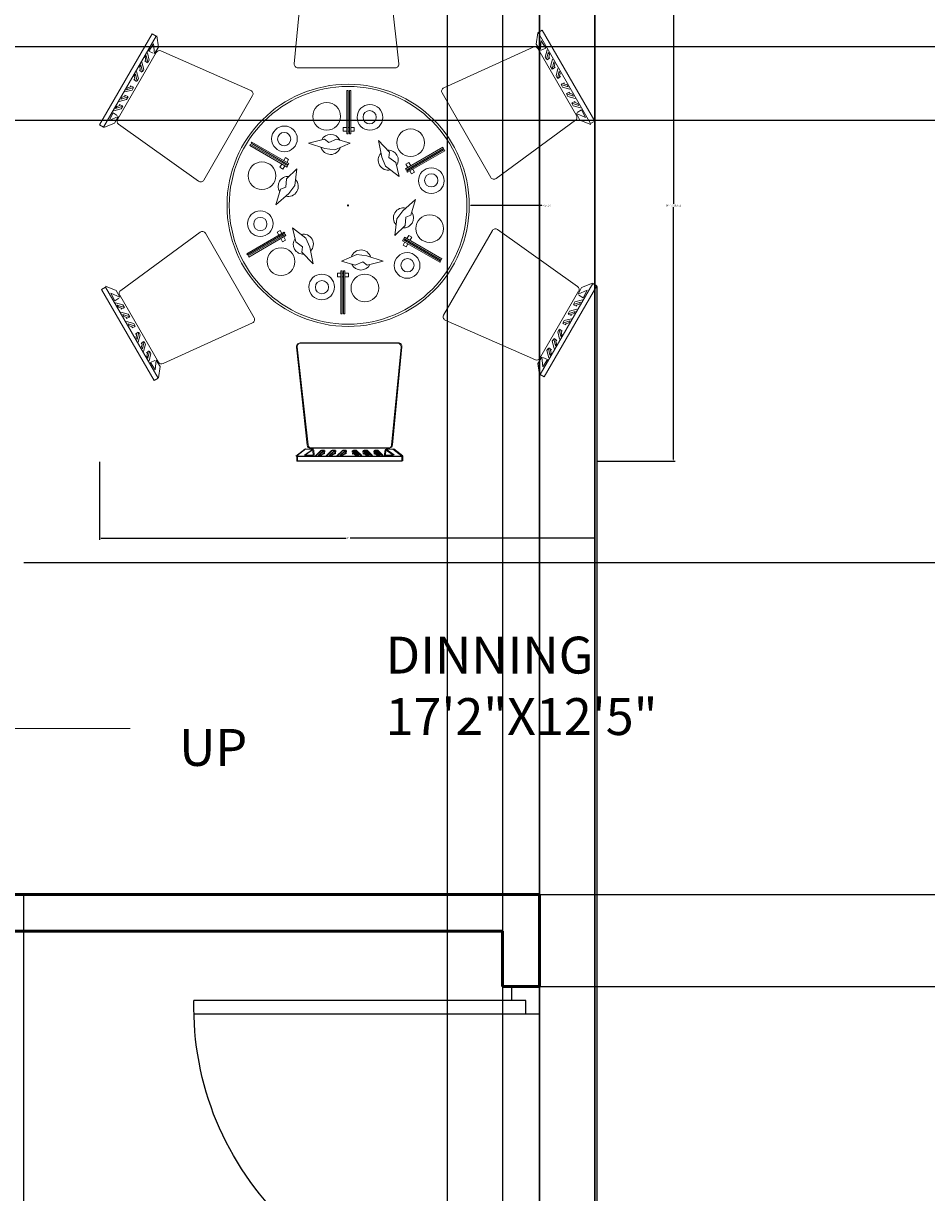
# Model space of a CAD drawing. Units: inches. Extents: x 1798 to 2141, y 1923 to 2386.
# Tile 3 of 9: x 1921 to 2019, y 2050 to 2177. Entities that reach past the tile are written whole.
import ezdxf

# ---------------------------------------------------------------- set-up
doc = ezdxf.new("R2010")
doc.units = ezdxf.units.IN
for name, color, linetype, lineweight in [('A-ANNO-DIMS', 2, 'Continuous', 18), ('A-ANNO-SYMB', 7, 'Continuous', 18), ('A-ANNO-TEXT', 7, 'Continuous', 18), ('A-AREA-IDEN', 7, 'Continuous', 25), ('A-FURN', 8, 'Continuous', 13), ('door', 40, 'Continuous', 25), ('wall', 4, 'Continuous', 50)]:
    doc.layers.add(name, color=color, linetype=linetype, lineweight=lineweight)
doc.styles.get("Standard").update_dxf_attribs({"font": 'arial.ttf'})
doc.dimstyles.get("Standard").update_dxf_attribs({"dimtxt": 0.18, "dimasz": 0.18, "dimexe": 0.18, "dimexo": 0.0625, "dimgap": 0.09, "dimtad": 0, "dimtih": 1, "dimtoh": 1, "dimdec": 4, "dimzin": 0, "dimdsep": 46, "dimtxsty": 'Standard', "dimcen": 0.09, "dimadec": 0, "dimazin": 0, "dimtfac": 1, "dimtdec": 4, "dimtofl": 0, "dimtmove": 0, "dimatfit": 3, "dimfxl": 1, "dimtolj": 1, "dimtzin": 0, "dimarcsym": 0})

# ---------------------------------------------------------------- blocks, each defined once
blk = doc.blocks.new('A$C45501D90')
for p, q in [((-242.2, 1133.5), (224, 1133.5)), ((-242.2, 1112.8), (-242.2, 1133.5)), ((224, 1112.8), (-242.2, 1112.8)), ((-242.2, 1111.2), (-202.3, 1079.2)), ((-203.9, 1106.4), (-165.6, 1108)), ((-168.8, 1080.8), (-203.9, 1106.4)), ((-165.6, 1108), (-167.2, 1085.6)), ((-156, 1109.6), (-132, 1085.6)), ((-119.3, 1085.6), (-143.2, 1108)), ((-143.2, 1108), (-133.6, 1108)), ((-133.6, 1108), (-122.5, 1098.4)), ((-122.5, 1098.4), (-119.3, 1101.6)), ((-119.3, 1101.6), (-117.7, 1087.2)), ((-108.1, 1109.6), (-84.1, 1085.6)), ((-71.4, 1085.6), (-95.3, 1108)), ((-95.3, 1108), (-85.7, 1108)), ((-85.7, 1108), (-74.6, 1098.4)), ((-74.6, 1098.4), (-71.4, 1101.6)), ((-71.4, 1101.6), (-69.8, 1087.2)), ((-60.2, 1109.6), (-36.2, 1085.6)), ((-23.5, 1085.6), (-47.4, 1108)), ((-47.4, 1108), (-37.8, 1108)), ((-37.8, 1108), (-26.7, 1098.4)), ((-26.7, 1098.4), (-23.5, 1101.6)), ((-23.5, 1101.6), (-21.9, 1087.2)), ((8.5, 1101.6), (6.9, 1087.2)), ((8.5, 1085.6), (32.4, 1108)), ((11.6, 1098.4), (8.5, 1101.6)), ((22.8, 1108), (11.6, 1098.4)), ((45.2, 1109.6), (21.2, 1085.6)), ((32.4, 1108), (22.8, 1108)), ((56.3, 1101.6), (54.8, 1087.2)), ((56.3, 1085.6), (80.3, 1108)), ((59.5, 1098.4), (56.3, 1101.6)), ((70.7, 1108), (59.5, 1098.4)), ((93.1, 1109.6), (69.1, 1085.6)), ((80.3, 1108), (70.7, 1108)), ((104.2, 1101.6), (102.6, 1087.2)), ((104.2, 1085.6), (128.2, 1108)), ((107.4, 1098.4), (104.2, 1101.6)), ((118.6, 1108), (107.4, 1098.4)), ((141, 1109.6), (117, 1085.6)), ((128.2, 1108), (118.6, 1108)), ((188.9, 1106.4), (150.5, 1108)), ((150.5, 1108), (152.1, 1085.6)), ((153.7, 1080.8), (188.9, 1106.4)), ((224, 1112.8), (187.3, 1079.2)), ((224, 1133.5), (224, 1112.8)), ((-197.3, 1061.6), (-238.9, 627.6)), ((-202.3, 1079.2), (-168.8, 1080.8)), ((161.8, 1076.1), (-181.4, 1076.1)), ((-132, 1085.6), (-119.3, 1085.6)), ((-84.1, 1085.6), (-71.4, 1085.6)), ((-36.2, 1085.6), (-23.5, 1085.6)), ((21.2, 1085.6), (8.5, 1085.6)), ((69.1, 1085.6), (56.3, 1085.6)), ((117, 1085.6), (104.2, 1085.6)), ((187.3, 1079.2), (153.7, 1080.8)), ((225.2, 627.8), (177.6, 1061.8)), ((-1102.7, 357), (-869.7, 760.7)), ((-851.7, 750.4), (-1084.8, 346.6)), ((-869.7, 760.7), (-851.7, 750.4)), ((-848.7, 752.3), (-841, 701.8)), ((841.2, 765.3), (833.5, 714.8)), ((842.6, 766.1), (860.5, 776.5)), ((1075.7, 362.4), (842.6, 766.1)), ((851.7, 686.6), (856.2, 729.8)), ((856.2, 729.8), (876.7, 697.4)), ((860.5, 776.5), (1093.6, 372.8)), ((-851, 678.1), (-1022.6, 380.9)), ((-890.4, 676.9), (-881.7, 644.2)), ((-863.7, 716.7), (-884.3, 684.4)), ((-884.3, 684.4), (-864.1, 674.6)), ((-859.2, 673.6), (-863.7, 716.7)), ((-841, 701.8), (-859.2, 673.6)), ((-431.1, 509), (-830.8, 684.8)), ((820.7, 701.7), (424.1, 520.7)), ((833.5, 714.8), (851.7, 686.6)), ((1012.8, 397.9), (841.2, 695.1)), ((876.7, 697.4), (856.6, 687.6)), ((882.9, 689.9), (874.2, 657.2)), ((880.6, 646.1), (887.9, 678)), ((887.9, 678), (892.7, 669.7)), ((-919.4, 623.5), (-924.2, 615.2)), ((-912, 591.6), (-919.4, 623.5)), ((-914.4, 635.4), (-905.6, 602.7)), ((-897.5, 642.2), (-901.9, 641.1)), ((-901.9, 641.1), (-890.2, 632.5)), ((-895.4, 665), (-900.2, 656.7)), ((-900.2, 656.7), (-897.5, 642.2)), ((-888.1, 633.1), (-895.4, 665)), ((-881.7, 644.2), (-888.1, 633.1)), ((874.2, 657.2), (880.6, 646.1)), ((894.4, 654.1), (882.7, 645.5)), ((892.7, 669.7), (890, 655.2)), ((890, 655.2), (894.4, 654.1)), ((906.9, 648.4), (898.1, 615.7)), ((904.5, 604.6), (911.9, 636.5)), ((911.9, 636.5), (916.7, 628.2)), ((916.7, 628.2), (914, 613.8)), ((-943.3, 582), (-948.1, 573.8)), ((-948.1, 573.8), (-945.4, 559.3)), ((-936, 550.1), (-943.3, 582)), ((-938.3, 593.9), (-929.6, 561.2)), ((-921.5, 600.8), (-925.8, 599.6)), ((-925.8, 599.6), (-914.2, 591)), ((-924.2, 615.2), (-921.5, 600.8)), ((-905.6, 602.7), (-912, 591.6)), ((-223, 610.1), (209.4, 610.1)), ((898.1, 615.7), (904.5, 604.6)), ((918.3, 612.6), (906.7, 604)), ((914, 613.8), (918.3, 612.6)), ((930.8, 606.9), (922.1, 574.2)), ((922.1, 574.2), (928.4, 563.1)), ((928.4, 563.1), (935.8, 595.1)), ((942.3, 571.1), (930.6, 562.6)), ((935.8, 595.1), (940.6, 586.8)), ((940.6, 586.8), (937.9, 572.3)), ((937.9, 572.3), (942.3, 571.1)), ((-951.9, 522.5), (-983.2, 512.9)), ((-983.2, 512.9), (-978.5, 521.2)), ((-978.5, 521.2), (-964.6, 526.1)), ((-964.6, 526.1), (-965.7, 530.5)), ((-965.7, 530.5), (-952.5, 524.7)), ((-958.3, 511.4), (-951.9, 522.5)), ((-945.4, 559.3), (-949.8, 558.1)), ((-949.8, 558.1), (-938.1, 549.6)), ((-929.6, 561.2), (-936, 550.1)), ((950.8, 524.4), (944.4, 535.5)), ((944.4, 535.5), (975.7, 525.9)), ((958.2, 543.5), (945, 537.7)), ((983.5, 515.7), (950.8, 524.4)), ((957.1, 539.1), (958.2, 543.5)), ((970.9, 534.2), (957.1, 539.1)), ((975.7, 525.9), (970.9, 534.2)), ((-1015, 461.2), (-982.3, 469.9)), ((-975.9, 481), (-1007.2, 471.4)), ((-1007.2, 471.4), (-1002.4, 479.7)), ((-1002.4, 479.7), (-988.5, 484.6)), ((-991, 502.7), (-958.3, 511.4)), ((-988.5, 484.6), (-989.7, 489)), ((-989.7, 489), (-976.5, 483.2)), ((-982.3, 469.9), (-975.9, 481)), ((-639.9, 111.9), (-423.7, 486.4)), ((-5.6, 508.7, 90.8), (0.4, 508.7, 90.8)), ((-5.6, 317.7, 90.8), (-5.6, 508.7, 90.8)), ((0.4, 508.7, 90.8), (0.4, 317.7, 90.8)), ((5.8, 317.7, 90.8), (5.8, 508.7, 90.8)), ((5.8, 508.7, 90.8), (11.8, 508.7, 90.8)), ((11.8, 508.7, 90.8), (11.8, 317.7, 90.8)), ((416.9, 498.2), (633.1, 123.7)), ((968.4, 494), (999.7, 484.4)), ((974.7, 483), (968.4, 494)), ((982.2, 502), (968.9, 496.2)), ((1007.4, 474.2), (974.7, 483)), ((981, 497.6), (982.2, 502)), ((994.9, 492.7), (981, 497.6)), ((999.7, 484.4), (994.9, 492.7)), ((-1038.9, 419.7), (-1006.2, 428.5)), ((-999.8, 439.5), (-1031.1, 430)), ((-1031.1, 430), (-1026.3, 438.3)), ((-1026.3, 438.3), (-1012.5, 443.1)), ((-1012.5, 443.1), (-1013.6, 447.5)), ((-1013.6, 447.5), (-1000.4, 441.7)), ((-1006.2, 428.5), (-999.8, 439.5)), ((998.7, 441.5), (992.3, 452.5)), ((992.3, 452.5), (1023.6, 443)), ((1006.1, 460.5), (992.9, 454.7)), ((1031.4, 432.7), (998.7, 441.5)), ((1005, 456.2), (1006.1, 460.5)), ((1018.8, 451.3), (1005, 456.2)), ((1034.8, 423.6), (1016.3, 411.1)), ((1023.6, 443), (1018.8, 451.3)), ((1052.6, 389.6), (1034.8, 423.6)), ((-1083.4, 345.8), (-1035.8, 364.4)), ((-1060.1, 376.6), (-1042.3, 410.6)), ((-1020.4, 394.3), (-1060.1, 376.6)), ((-1042.3, 410.6), (-1023.8, 398.1)), ((-1035.8, 364.4), (-1020.4, 394.3)), ((656.3, 118.9), (1008.4, 377.1)), ((1028.3, 377.5), (1012.9, 407.3)), ((1012.9, 407.3), (1052.6, 389.6)), ((1075.9, 358.8), (1028.3, 377.5)), ((1093.6, 372.8), (1075.7, 362.4)), ((-1084.8, 346.6), (-1102.7, 357)), ((-1018, 360), (-663, 106.9)), ((-22.3, 329.1, 90.8), (-22.3, 344.6, 90.8)), ((-22.3, 344.6, 90.8), (-5.6, 344.6, 90.8)), ((-5.6, 329.1, 90.8), (-22.3, 329.1, 90.8)), ((0.4, 317.7, 90.8), (-5.6, 317.7, 90.8)), ((0.4, 344.6, 90.8), (5.8, 344.6, 90.8)), ((5.8, 329.1, 90.8), (0.4, 329.1, 90.8)), ((11.8, 317.7, 90.8), (5.8, 317.7, 90.8)), ((11.8, 344.6, 90.8), (27.3, 344.6, 90.8)), ((27.3, 329.1, 90.8), (11.8, 329.1, 90.8)), ((27.3, 344.6, 90.8), (27.3, 329.1, 90.8)), ((-436.3, 265.3, 90.8), (-433.3, 270.5, 90.8)), ((-270.9, 169.9, 90.8), (-436.3, 265.3, 90.8)), ((-433.3, 270.5, 90.8), (-267.9, 175, 90.8)), ((-430.6, 275.2, 90.8), (-427.6, 280.3, 90.8)), ((-265.2, 179.7, 90.8), (-430.6, 275.2, 90.8)), ((-427.6, 280.3, 90.8), (-262.3, 184.9, 90.8)), ((-175.3, 276.1, 90.8), (-104.8, 293.2, 90.8)), ((-103.3, 252.4, 90.8), (-175.3, 276.1, 90.8)), ((-104.8, 293.2, 90.8), (-85.5, 278.4, 90.8)), ((-85.5, 278.4, 90.8), (-52.1, 293.9, 90.8)), ((9.5, 276.1, 90.8), (-59.5, 246.5, 90.8)), ((-52.1, 293.9, 90.8), (9.5, 276.1, 90.8)), ((134.3, 288, 90.8), (184.3, 235.5, 90.8)), ((149.7, 213.9, 90.8), (134.3, 288, 90.8)), ((-285.5, 198.3, 90.8), (-277.8, 211.7, 90.8)), ((-277.8, 211.7, 90.8), (-264.3, 204, 90.8)), ((-59.5, 246.5, 90.8), (-103.3, 252.4, 90.8)), ((166.5, 173, 90.8), (149.7, 213.9, 90.8)), ((184.3, 235.5, 90.8), (181.1, 211.4, 90.8)), ((181.1, 211.4, 90.8), (211.3, 190.3, 90.8)), ((255.2, 161.9, 90.8), (420.6, 257.3, 90.8)), ((423.5, 252.2, 90.8), (258.2, 156.7, 90.8)), ((260.9, 152, 90.8), (426.2, 247.5, 90.8)), ((429.2, 242.3, 90.8), (263.8, 146.9, 90.8)), ((420.6, 257.3, 90.8), (423.5, 252.2, 90.8)), ((426.2, 247.5, 90.8), (429.2, 242.3, 90.8)), ((-302.5, 168.8, 90.8), (-294.2, 183.3, 90.8)), ((-289.1, 161.1, 90.8), (-302.5, 168.8, 90.8)), ((-291.2, 188.5, 90.8), (-288.5, 193.1, 90.8)), ((-280.7, 175.5, 90.8), (-289.1, 161.1, 90.8)), ((-275.1, 185.4, 90.8), (-277.8, 180.7, 90.8)), ((-273.6, 117.6, 90.8), (-227.4, 162.1, 90.8)), ((-264.3, 204, 90.8), (-272.1, 190.5, 90.8)), ((-267.9, 175, 90.8), (-270.9, 169.9, 90.8)), ((-262.3, 184.9, 90.8), (-265.2, 179.7, 90.8)), ((-227.4, 162.1, 90.8), (-236.2, 87.5, 90.8)), ((226.7, 128.1, 90.8), (166.5, 173, 90.8)), ((211.3, 190.3, 90.8), (226.7, 128.1, 90.8)), ((258.2, 156.7, 90.8), (255.2, 161.9, 90.8)), ((256.6, 182, 90.8), (270.1, 189.8, 90.8)), ((265, 167.5, 90.8), (256.6, 182, 90.8)), ((270.7, 157.7, 90.8), (268, 162.4, 90.8)), ((270.1, 189.8, 90.8), (278.4, 175.3, 90.8)), ((281.4, 170.1, 90.8), (284.1, 165.5, 90.8)), ((287.1, 160.3, 90.8), (294.9, 146.8, 90.8)), ((-276.8, 80.9, 90.8), (-273.6, 117.6, 90.8)), ((263.8, 146.9, 90.8), (260.9, 152, 90.8)), ((281.4, 139.1, 90.8), (273.7, 152.5, 90.8)), ((294.9, 146.8, 90.8), (281.4, 139.1, 90.8)), ((-319.8, 2.1, 90.8), (-299.3, 71.7, 90.8)), ((-263.2, 52.5, 90.8), (-319.8, 2.1, 90.8)), ((-299.3, 71.7, 90.8), (-276.8, 80.9, 90.8)), ((-236.2, 87.5, 90.8), (-263.2, 52.5, 90.8)), ((242.9, -24.6, 90.8), (299.4, 25.9, 90.8)), ((299.4, 25.9, 90.8), (278.9, -43.7, 90.8)), ((215.8, -59.5, 90.8), (242.9, -24.6, 90.8)), ((278.9, -43.7, 90.8), (256.4, -53, 90.8)), ((-247, -100.1, 90.8), (-186.8, -145, 90.8)), ((-231.7, -162.3, 90.8), (-247, -100.1, 90.8)), ((207, -134.1, 90.8), (215.8, -59.5, 90.8)), ((253.2, -89.7, 90.8), (207, -134.1, 90.8)), ((256.4, -53, 90.8), (253.2, -89.7, 90.8)), ((-656.3, -118.9), (-1008.4, -377.1)), ((-416.9, -498.2), (-633.1, -123.7)), ((-449.6, -214.4, 90.8), (-284.2, -118.9, 90.8)), ((-281.2, -124.1, 90.8), (-446.6, -219.5, 90.8)), ((-443.9, -224.2, 90.8), (-278.5, -128.7, 90.8)), ((-275.5, -133.9, 90.8), (-440.9, -229.4, 90.8)), ((-315.2, -118.9, 90.8), (-301.8, -111.1, 90.8)), ((-307.5, -132.3, 90.8), (-315.2, -118.9, 90.8)), ((-301.8, -142.1, 90.8), (-304.5, -137.5, 90.8)), ((-301.8, -111.1, 90.8), (-294, -124.6, 90.8)), ((-290.4, -161.8, 90.8), (-298.8, -147.3, 90.8)), ((-291, -129.7, 90.8), (-288.3, -134.4, 90.8)), ((-277, -154, 90.8), (-290.4, -161.8, 90.8)), ((-285.4, -139.5, 90.8), (-277, -154, 90.8)), ((-284.2, -118.9, 90.8), (-281.2, -124.1, 90.8)), ((-278.5, -128.7, 90.8), (-275.5, -133.9, 90.8)), ((-186.8, -145, 90.8), (-170.1, -185.9, 90.8)), ((241.9, -156.9, 90.8), (244.9, -151.7, 90.8)), ((244.9, -151.7, 90.8), (410.3, -247.2, 90.8)), ((247.6, -147.1, 90.8), (250.6, -141.9, 90.8)), ((413, -242.5, 90.8), (247.6, -147.1, 90.8)), ((250.6, -141.9, 90.8), (415.9, -237.4, 90.8)), ((254.7, -157.4, 90.8), (257.4, -152.7, 90.8)), ((260.4, -147.6, 90.8), (268.7, -133.1, 90.8)), ((268.7, -133.1, 90.8), (282.2, -140.8, 90.8)), ((282.2, -140.8, 90.8), (273.8, -155.3, 90.8)), ((639.9, -111.9), (423.7, -486.4)), ((1018, -360), (663, -106.9)), ((-201.5, -183.4, 90.8), (-231.7, -162.3, 90.8)), ((-204.7, -207.6, 90.8), (-201.5, -183.4, 90.8)), ((-170.1, -185.9, 90.8), (-154.7, -260.1, 90.8)), ((407.3, -252.4, 90.8), (241.9, -156.9, 90.8)), ((244, -176, 90.8), (251.7, -162.5, 90.8)), ((257.4, -183.7, 90.8), (244, -176, 90.8)), ((265.2, -170.3, 90.8), (257.4, -183.7, 90.8)), ((270.8, -160.5, 90.8), (268.1, -165.1, 90.8)), ((-446.6, -219.5, 90.8), (-449.6, -214.4, 90.8)), ((-440.9, -229.4, 90.8), (-443.9, -224.2, 90.8)), ((-154.7, -260.1, 90.8), (-204.7, -207.6, 90.8)), ((-29.8, -248.2, 90.8), (39.2, -218.5, 90.8)), ((31.8, -266, 90.8), (-29.8, -248.2, 90.8)), ((65.2, -250.4, 90.8), (31.8, -266, 90.8)), ((39.2, -218.5, 90.8), (83, -224.4, 90.8)), ((84.4, -265.2, 90.8), (65.2, -250.4, 90.8)), ((83, -224.4, 90.8), (154.9, -248.2, 90.8)), ((154.9, -248.2, 90.8), (84.4, -265.2, 90.8)), ((410.3, -247.2, 90.8), (407.3, -252.4, 90.8)), ((415.9, -237.4, 90.8), (413, -242.5, 90.8)), ((-47.6, -316.6, 90.8), (-47.6, -301.1, 90.8)), ((-47.6, -301.1, 90.8), (-32.1, -301.1, 90.8)), ((-32.1, -480.7, 90.8), (-32.1, -289.8, 90.8)), ((-32.1, -289.8, 90.8), (-26.1, -289.8, 90.8)), ((-26.1, -289.8, 90.8), (-26.1, -480.7, 90.8)), ((-26.1, -301.1, 90.8), (-20.8, -301.1, 90.8)), ((-20.8, -480.7, 90.8), (-20.8, -289.8, 90.8)), ((-20.8, -289.8, 90.8), (-14.8, -289.8, 90.8)), ((-14.8, -289.8, 90.8), (-14.8, -480.7, 90.8)), ((-14.8, -301.1, 90.8), (1.9, -301.1, 90.8)), ((1.9, -301.1, 90.8), (1.9, -316.6, 90.8)), ((-1093.6, -372.8), (-1075.7, -362.4)), ((-1075.9, -358.8), (-1028.3, -377.5)), ((-1075.7, -362.4), (-842.6, -766.1)), ((-32.1, -316.6, 90.8), (-47.6, -316.6, 90.8)), ((-20.8, -316.6, 90.8), (-26.1, -316.6, 90.8)), ((1.9, -316.6, 90.8), (-14.8, -316.6, 90.8)), ((851.7, -750.4), (1084.8, -346.6)), ((1102.7, -357), (869.7, -760.7)), ((1083.4, -345.8), (1035.8, -364.4)), ((1084.8, -346.6), (1102.7, -357)), ((-860.5, -776.5), (-1093.6, -372.8)), ((-1052.6, -389.6), (-1034.8, -423.6)), ((-1012.9, -407.3), (-1052.6, -389.6)), ((-1034.8, -423.6), (-1016.3, -411.1)), ((-1028.3, -377.5), (-1012.9, -407.3)), ((-1012.8, -397.9), (-841.2, -695.1)), ((851, -678.1), (1022.6, -380.9)), ((1035.8, -364.4), (1020.4, -394.3)), ((1020.4, -394.3), (1060.1, -376.6)), ((1042.3, -410.6), (1023.8, -398.1)), ((1060.1, -376.6), (1042.3, -410.6)), ((-1031.4, -432.7), (-998.7, -441.5)), ((-1023.6, -443), (-1018.8, -451.3)), ((-992.3, -452.5), (-1023.6, -443)), ((-1018.8, -451.3), (-1005, -456.2)), ((-1006.1, -460.5), (-992.9, -454.7)), ((-1005, -456.2), (-1006.1, -460.5)), ((-998.7, -441.5), (-992.3, -452.5)), ((1015, -461.2), (982.3, -469.9)), ((1006.2, -428.5), (999.8, -439.5)), ((999.8, -439.5), (1031.1, -430)), ((1013.6, -447.5), (1000.4, -441.7)), ((1038.9, -419.7), (1006.2, -428.5)), ((1026.3, -438.3), (1012.5, -443.1)), ((1012.5, -443.1), (1013.6, -447.5)), ((1031.1, -430), (1026.3, -438.3)), ((-1007.4, -474.2), (-974.7, -483)), ((-968.4, -494), (-999.7, -484.4)), ((-999.7, -484.4), (-994.9, -492.7)), ((-994.9, -492.7), (-981, -497.6)), ((-983.5, -515.7), (-950.8, -524.4)), ((-982.2, -502), (-968.9, -496.2)), ((-981, -497.6), (-982.2, -502)), ((-974.7, -483), (-968.4, -494)), ((-26.1, -480.7, 90.8), (-32.1, -480.7, 90.8)), ((-14.8, -480.7, 90.8), (-20.8, -480.7, 90.8)), ((431.1, -509), (830.8, -684.8)), ((958.3, -511.4), (951.9, -522.5)), ((951.9, -522.5), (983.2, -512.9)), ((991, -502.7), (958.3, -511.4)), ((982.3, -469.9), (975.9, -481)), ((975.9, -481), (1007.2, -471.4)), ((989.7, -489), (976.5, -483.2)), ((983.2, -512.9), (978.5, -521.2)), ((1002.4, -479.7), (988.5, -484.6)), ((988.5, -484.6), (989.7, -489)), ((1007.2, -471.4), (1002.4, -479.7)), ((-944.4, -535.5), (-975.7, -525.9)), ((-975.7, -525.9), (-970.9, -534.2)), ((-970.9, -534.2), (-957.1, -539.1)), ((-958.2, -543.5), (-945, -537.7)), ((-957.1, -539.1), (-958.2, -543.5)), ((-950.8, -524.4), (-944.4, -535.5)), ((-942.3, -571.1), (-930.6, -562.6)), ((-928.4, -563.1), (-935.8, -595.1)), ((-922.1, -574.2), (-928.4, -563.1)), ((-820.7, -701.7), (-424.1, -520.7)), ((929.6, -561.2), (936, -550.1)), ((938.3, -593.9), (929.6, -561.2)), ((936, -550.1), (943.3, -582)), ((949.8, -558.1), (938.1, -549.6)), ((945.4, -559.3), (949.8, -558.1)), ((948.1, -573.8), (945.4, -559.3)), ((965.7, -530.5), (952.5, -524.7)), ((978.5, -521.2), (964.6, -526.1)), ((964.6, -526.1), (965.7, -530.5)), ((-937.9, -572.3), (-942.3, -571.1)), ((-940.6, -586.8), (-937.9, -572.3)), ((-935.8, -595.1), (-940.6, -586.8)), ((-930.8, -606.9), (-922.1, -574.2)), ((-918.3, -612.6), (-906.7, -604)), ((-914, -613.8), (-918.3, -612.6)), ((-916.7, -628.2), (-914, -613.8)), ((-904.5, -604.6), (-911.9, -636.5)), ((-906.9, -648.4), (-898.1, -615.7)), ((-898.1, -615.7), (-904.5, -604.6)), ((218.9, -611.6), (-213.5, -611.6)), ((223, -610.1), (-209.4, -610.1)), ((905.6, -602.7), (912, -591.6)), ((914.4, -635.4), (905.6, -602.7)), ((912, -591.6), (919.4, -623.5)), ((925.8, -599.6), (914.2, -591)), ((919.4, -623.5), (924.2, -615.2)), ((921.5, -600.8), (925.8, -599.6)), ((924.2, -615.2), (921.5, -600.8)), ((943.3, -582), (948.1, -573.8)), ((-911.9, -636.5), (-916.7, -628.2)), ((-894.4, -654.1), (-882.7, -645.5)), ((-890, -655.2), (-894.4, -654.1)), ((-892.7, -669.7), (-890, -655.2)), ((-887.9, -678), (-892.7, -669.7)), ((-880.6, -646.1), (-887.9, -678)), ((-882.9, -689.9), (-874.2, -657.2)), ((-874.2, -657.2), (-880.6, -646.1)), ((-229.3, -629.3), (-181.8, -1063.3)), ((-225.2, -627.8), (-177.6, -1061.8)), ((193.2, -1063.1), (234.8, -629.1)), ((197.3, -1061.6), (238.9, -627.6)), ((841, -701.8), (859.2, -673.6)), ((859.2, -673.6), (863.7, -716.7)), ((881.7, -644.2), (888.1, -633.1)), ((890.4, -676.9), (881.7, -644.2)), ((888.1, -633.1), (895.4, -665)), ((901.9, -641.1), (890.2, -632.5)), ((895.4, -665), (900.2, -656.7)), ((897.5, -642.2), (901.9, -641.1)), ((900.2, -656.7), (897.5, -642.2)), ((-876.7, -697.4), (-856.6, -687.6)), ((-856.2, -729.8), (-876.7, -697.4)), ((-851.7, -686.6), (-856.2, -729.8)), ((-833.5, -714.8), (-851.7, -686.6)), ((-841.2, -765.3), (-833.5, -714.8)), ((848.7, -752.3), (841, -701.8)), ((863.7, -716.7), (884.3, -684.4)), ((884.3, -684.4), (864.1, -674.6)), ((-842.6, -766.1), (-860.5, -776.5)), ((869.7, -760.7), (851.7, -750.4)), ((-231.3, -1112.7), (-191.4, -1080.8)), ((-227.2, -1111.2), (-187.3, -1079.2)), ((-157.9, -1082.4), (-193, -1107.9)), ((-191.4, -1080.8), (-157.9, -1082.4)), ((-153.7, -1080.8), (-188.9, -1106.4)), ((-187.3, -1079.2), (-153.7, -1080.8)), ((-165.9, -1077.6), (177.3, -1077.6)), ((-161.8, -1076.1), (181.4, -1076.1)), ((-154.7, -1109.5), (-156.3, -1087.1)), ((-150.5, -1108), (-152.1, -1085.6)), ((-145.1, -1111.1), (-121.1, -1087.1)), ((-141, -1109.6), (-117, -1085.6)), ((-108.4, -1087.1), (-132.3, -1109.5)), ((-104.2, -1085.6), (-128.2, -1108)), ((-121.1, -1087.1), (-108.4, -1087.1)), ((-117, -1085.6), (-104.2, -1085.6)), ((-108.4, -1103.1), (-106.8, -1088.7)), ((-104.2, -1101.6), (-102.6, -1087.2)), ((-97.2, -1111.1), (-73.2, -1087.1)), ((-93.1, -1109.6), (-69.1, -1085.6)), ((-60.5, -1087.1), (-84.4, -1109.5)), ((-56.3, -1085.6), (-80.3, -1108)), ((-73.2, -1087.1), (-60.5, -1087.1)), ((-69.1, -1085.6), (-56.3, -1085.6)), ((-60.5, -1103.1), (-58.9, -1088.7)), ((-56.3, -1101.6), (-54.8, -1087.2)), ((-49.3, -1111.1), (-25.3, -1087.1)), ((-45.2, -1109.6), (-21.2, -1085.6)), ((-12.6, -1087.1), (-36.5, -1109.5)), ((-8.5, -1085.6), (-32.4, -1108)), ((-25.3, -1087.1), (-12.6, -1087.1)), ((-21.2, -1085.6), (-8.5, -1085.6)), ((-12.6, -1103.1), (-11, -1088.7)), ((-8.5, -1101.6), (-6.9, -1087.2)), ((19.4, -1103.1), (17.8, -1088.7)), ((19.4, -1087.1), (43.3, -1109.5)), ((32.1, -1087.1), (19.4, -1087.1)), ((23.5, -1101.6), (21.9, -1087.2)), ((23.5, -1085.6), (47.4, -1108)), ((36.2, -1085.6), (23.5, -1085.6)), ((56.1, -1111.1), (32.1, -1087.1)), ((60.2, -1109.6), (36.2, -1085.6)), ((67.3, -1103.1), (65.7, -1088.7)), ((67.3, -1087.1), (91.2, -1109.5)), ((80, -1087.1), (67.3, -1087.1)), ((71.4, -1101.6), (69.8, -1087.2)), ((71.4, -1085.6), (95.3, -1108)), ((84.1, -1085.6), (71.4, -1085.6)), ((104, -1111.1), (80, -1087.1)), ((108.1, -1109.6), (84.1, -1085.6)), ((115.1, -1103.1), (113.6, -1088.7)), ((115.1, -1087.1), (139.1, -1109.5)), ((127.9, -1087.1), (115.1, -1087.1)), ((119.3, -1101.6), (117.7, -1087.2)), ((119.3, -1085.6), (143.2, -1108)), ((132, -1085.6), (119.3, -1085.6)), ((151.9, -1111.1), (127.9, -1087.1)), ((156, -1109.6), (132, -1085.6)), ((161.4, -1109.5), (163, -1087.1)), ((198.2, -1080.8), (164.6, -1082.4)), ((164.6, -1082.4), (199.8, -1107.9)), ((165.6, -1108), (167.2, -1085.6)), ((202.3, -1079.2), (168.8, -1080.8)), ((168.8, -1080.8), (203.9, -1106.4)), ((238.1, -1112.7), (198.2, -1080.8)), ((242.2, -1111.2), (202.3, -1079.2)), ((-228.1, -1114.3), (238.1, -1114.3)), ((-228.1, -1135), (-228.1, -1114.3)), ((238.1, -1135), (-228.1, -1135)), ((-224, -1112.8), (242.2, -1112.8)), ((-224, -1133.5), (-224, -1112.8)), ((242.2, -1133.5), (-224, -1133.5)), ((-193, -1107.9), (-154.7, -1109.5)), ((-188.9, -1106.4), (-150.5, -1108)), ((-132.3, -1109.5), (-122.7, -1109.5)), ((-128.2, -1108), (-118.6, -1108)), ((-122.7, -1109.5), (-111.6, -1099.9)), ((-118.6, -1108), (-107.4, -1098.4)), ((-111.6, -1099.9), (-108.4, -1103.1)), ((-107.4, -1098.4), (-104.2, -1101.6)), ((-84.4, -1109.5), (-74.8, -1109.5)), ((-80.3, -1108), (-70.7, -1108)), ((-74.8, -1109.5), (-63.7, -1099.9)), ((-70.7, -1108), (-59.5, -1098.4)), ((-63.7, -1099.9), (-60.5, -1103.1)), ((-59.5, -1098.4), (-56.3, -1101.6)), ((-36.5, -1109.5), (-26.9, -1109.5)), ((-32.4, -1108), (-22.8, -1108)), ((-26.9, -1109.5), (-15.8, -1099.9)), ((-22.8, -1108), (-11.6, -1098.4)), ((-15.8, -1099.9), (-12.6, -1103.1)), ((-11.6, -1098.4), (-8.5, -1101.6)), ((22.6, -1099.9), (19.4, -1103.1)), ((33.7, -1109.5), (22.6, -1099.9)), ((26.7, -1098.4), (23.5, -1101.6)), ((37.8, -1108), (26.7, -1098.4)), ((43.3, -1109.5), (33.7, -1109.5)), ((47.4, -1108), (37.8, -1108)), ((70.4, -1099.9), (67.3, -1103.1)), ((81.6, -1109.5), (70.4, -1099.9)), ((74.6, -1098.4), (71.4, -1101.6)), ((85.7, -1108), (74.6, -1098.4)), ((91.2, -1109.5), (81.6, -1109.5)), ((95.3, -1108), (85.7, -1108)), ((118.3, -1099.9), (115.1, -1103.1)), ((129.5, -1109.5), (118.3, -1099.9)), ((122.5, -1098.4), (119.3, -1101.6)), ((133.6, -1108), (122.5, -1098.4)), ((139.1, -1109.5), (129.5, -1109.5)), ((143.2, -1108), (133.6, -1108)), ((199.8, -1107.9), (161.4, -1109.5)), ((203.9, -1106.4), (165.6, -1108)), ((238.1, -1114.3), (238.1, -1135)), ((242.2, -1112.8), (242.2, -1133.5))]:
    blk.add_line(p, q)
for centre, radius in [((0, 0), 537), ((0, 0), 527), ((-94.8, 394.7, 90.8), 61.3), ((96.9, 390, 90.8), 56.9), ((95.5, 390.7, 90.8), 29.4), ((-282.3, 294.7, 90.8), 56.9), ((-283.5, 293.9, 90.8), 29.4), ((277.2, 277.6, 90.8), 61.3), ((-382.1, 131.1, 90.8), 61.3), ((369, 109.3, 90.8), 56.9), ((368.9, 110.8, 90.8), 29.4), ((-389.3, -81.3, 90.8), 56.9), ((361.8, -103.1, 90.8), 61.3), ((-389.2, -82.8, 90.8), 29.4), ((-297.5, -249.6, 90.8), 61.3), ((261.9, -266.7, 90.8), 56.9), ((263.2, -265.9, 90.8), 29.4), ((-117.2, -362, 90.8), 56.9), ((74.4, -366.7, 90.8), 61.3), ((-115.9, -362.7, 90.8), 29.4)]:
    blk.add_circle(centre, radius)
for centre, radius, start, end in [((-181.4, 1060.1), 16, 90, 174.5199), ((161.8, 1060.1), 16, 6.2572, 90), ((-837.2, 670.1), 16, 66.2572, 150), ((827.4, 687.1), 16, 30, 114.5199), ((-223, 626.1), 16, 174.5199, 270), ((209.4, 626.1), 16, 270, 6.2572), ((430.7, 506.2), 16, 114.5199, 210), ((-437.5, 494.4), 16, 330, 66.2572), ((-1008.8, 373), 16, 150, 234.5199), ((999, 389.9), 16, 306.2572, 30), ((-77.3, 270.2, 90.8), 44.6, 25.8558, 153.3359), ((-77.3, 270.2, 90.8), 44.6, 195.9338, 342.9389), ((178.1, 200.3, 90.8), 44.6, 135.9338, 282.9389), ((178.1, 200.3, 90.8), 44.6, 325.8558, 93.3359), ((-653.7, 119.9), 16, 234.5199, 330), ((-265.7, 83.9, 90.8), 44.6, 85.8558, 213.3359), ((-265.7, 83.9, 90.8), 44.6, 255.9338, 42.9389), ((646.9, 131.7), 16, 210, 306.2572), ((245.3, -55.9, 90.8), 44.6, 75.9338, 222.9389), ((245.3, -55.9, 90.8), 44.6, 265.8558, 33.3359), ((-646.9, -131.7), 16, 30, 126.2572), ((-198.5, -172.3, 90.8), 44.6, 145.8558, 273.3359), ((-198.5, -172.3, 90.8), 44.6, 315.9338, 102.9389), ((653.7, -119.9), 16, 54.5199, 150), ((57, -242.2, 90.8), 44.6, 15.9338, 162.9389), ((57, -242.2, 90.8), 44.6, 205.8558, 333.3359), ((1008.8, -373), 16, 330, 54.5199), ((-999, -389.9), 16, 126.2572, 210), ((-430.7, -506.2), 16, 294.5199, 30), ((437.5, -494.4), 16, 150, 246.2572), ((-213.5, -627.6), 16, 90, 186.2572), ((-209.4, -626.1), 16, 90, 186.2572), ((218.9, -627.6), 16, 354.5199, 90), ((223, -626.1), 16, 354.5199, 90), ((-827.4, -687.1), 16, 210, 294.5199), ((837.2, -670.1), 16, 246.2572, 330), ((-165.9, -1061.6), 16, 186.2572, 270), ((-161.8, -1060.1), 16, 186.2572, 270), ((177.3, -1061.6), 16, 270, 354.5199), ((181.4, -1060.1), 16, 270, 354.5199)]:
    blk.add_arc(centre, radius, start, end)
blk = doc.blocks.new('DOOR-SWING-36IN')
for p, q in [((1.5, 1.5), (1.5, 37.5)), ((3, 1.5), (3, 37.5)), ((0, 3), (0, 0)), ((1.5, 3), (0, 3)), ((1.5, 1.5), (1.5, 3)), ((34.5, 1.5), (34.5, 3)), ((34.5, 3), (36, 3)), ((36, 3), (36, 0)), ((3, 1.5), (1.5, 1.5)), ((3, 0), (3, 1.5)), ((33, 0), (33, 1.5)), ((33, 1.5), (34.5, 1.5)), ((0, 0), (3, 0)), ((36, 0), (33, 0))]:
    blk.add_line(p, q)
blk.add_arc((2.25, 5.18), 32.32, 356.1244, 91.3295)
blk = doc.blocks.new('*D23')
at = {"layer": 'A-ANNO-DIMS', "color": 0, "lineweight": -2, "transparency": 16777216}
for p, q in [((1982.78, 2184.81), (1991.23, 2184.81)), ((1991.05, 2184.63), (1991.05, 2157.25)), ((1991.05, 2129.5), (1991.05, 2156.88)), ((1982.78, 2129.32), (1991.23, 2129.32))]:
    blk.add_line(p, q, dxfattribs=at)
at = {"layer": 'A-ANNO-DIMS', "color": 0, "transparency": 16777216}
for points in [[(1991.02, 2184.63), (1991.08, 2184.63), (1991.05, 2184.81)], [(1991.02, 2129.5), (1991.08, 2129.5), (1991.05, 2129.32)]]:
    blk.add_solid(points, dxfattribs=at)
at = {"layer": 'Defpoints', "color": 0, "transparency": 16777216}
for p in [(1982.72, 2184.81), (1991.05, 2184.81), (1982.72, 2129.32)]:
    blk.add_point(p, dxfattribs=at)
at = {"layer": 'A-ANNO-DIMS', "color": 0, "transparency": 16777216, "insert": (1991.05, 2157.07), "char_height": 0.18, "attachment_point": 5}
blk.add_mtext('\\A1;DINING SET 55', dxfattribs=at)
blk = doc.blocks.new('*D24')
at = {"layer": 'A-ANNO-DIMS', "color": 0, "lineweight": -2, "transparency": 16777216}
for p, q in [((1928.77, 2129.25), (1928.77, 2120.81)), ((1982.72, 2129.25), (1982.72, 2120.81)), ((1928.95, 2120.99), (1955.53, 2120.99)), ((1982.54, 2120.99), (1955.96, 2120.99))]:
    blk.add_line(p, q, dxfattribs=at)
at = {"layer": 'A-ANNO-DIMS', "color": 0, "transparency": 16777216}
for points in [[(1928.95, 2121.02), (1928.95, 2120.96), (1928.77, 2120.99)], [(1982.54, 2121.02), (1982.54, 2120.96), (1982.72, 2120.99)]]:
    blk.add_solid(points, dxfattribs=at)
at = {"layer": 'Defpoints', "color": 0, "transparency": 16777216}
for p in [(1928.77, 2129.32), (1982.72, 2129.32), (1982.72, 2120.99)]:
    blk.add_point(p, dxfattribs=at)
at = {"layer": 'A-ANNO-DIMS', "color": 0, "transparency": 16777216, "insert": (1955.75, 2120.99), "char_height": 0.18, "attachment_point": 5}
blk.add_mtext('\\A1;54', dxfattribs=at)
blk = doc.blocks.new('*D35')
at = {"layer": 'A-ANNO-DIMS', "color": 0, "lineweight": -2, "transparency": 16777216}
for p, q in [((1972.51, 2235.26), (1972.51, 1923.12)), ((1966.51, 2231.26), (1966.51, 1923.12)), ((1966.69, 1923.3), (1969.36, 1923.3)), ((1972.33, 1923.3), (1969.66, 1923.3))]:
    blk.add_line(p, q, dxfattribs=at)
at = {"layer": 'A-ANNO-DIMS', "color": 0, "transparency": 16777216}
for points in [[(1966.69, 1923.33), (1966.69, 1923.27), (1966.51, 1923.3)], [(1972.33, 1923.33), (1972.33, 1923.27), (1972.51, 1923.3)]]:
    blk.add_solid(points, dxfattribs=at)
at = {"layer": 'Defpoints', "color": 0, "transparency": 16777216}
for p in [(1972.51, 2235.32), (1966.51, 2231.32), (1972.51, 1923.3)]:
    blk.add_point(p, dxfattribs=at)
at = {"layer": 'A-ANNO-DIMS', "color": 0, "transparency": 16777216, "insert": (1969.51, 1923.3), "char_height": 0.18, "attachment_point": 5}
blk.add_mtext('\\A1;6', dxfattribs=at)
blk = doc.blocks.new('*D36')
at = {"layer": 'A-ANNO-DIMS', "color": 0, "lineweight": -2, "transparency": 16777216}
for p, q in [((1976.51, 2231.26), (1976.51, 1923.12)), ((1982.51, 2231.26), (1982.51, 1923.12)), ((1976.69, 1923.3), (1979.36, 1923.3)), ((1982.33, 1923.3), (1979.66, 1923.3))]:
    blk.add_line(p, q, dxfattribs=at)
at = {"layer": 'A-ANNO-DIMS', "color": 0, "transparency": 16777216}
for points in [[(1976.69, 1923.33), (1976.69, 1923.27), (1976.51, 1923.3)], [(1982.33, 1923.33), (1982.33, 1923.27), (1982.51, 1923.3)]]:
    blk.add_solid(points, dxfattribs=at)
at = {"layer": 'Defpoints', "color": 0, "transparency": 16777216}
for p in [(1976.51, 2231.32), (1982.51, 2231.32), (1982.51, 1923.3)]:
    blk.add_point(p, dxfattribs=at)
at = {"layer": 'A-ANNO-DIMS', "color": 0, "transparency": 16777216, "insert": (1979.51, 1923.3), "char_height": 0.18, "attachment_point": 5}
blk.add_mtext('\\A1;6', dxfattribs=at)
blk = doc.blocks.new('*D39')
at = {"layer": 'A-ANNO-DIMS', "color": 0, "lineweight": -2, "transparency": 16777216}
for p, q in [((1976.51, 2035.39), (1976.51, 2385.53)), ((1976.69, 2385.35), (1979.36, 2385.35)), ((1982.33, 2385.35), (1979.66, 2385.35)), ((1982.51, 2035.39), (1982.51, 2385.53))]:
    blk.add_line(p, q, dxfattribs=at)
at = {"layer": 'A-ANNO-DIMS', "color": 0, "transparency": 16777216}
for points in [[(1976.69, 2385.38), (1976.69, 2385.32), (1976.51, 2385.35)], [(1982.33, 2385.38), (1982.33, 2385.32), (1982.51, 2385.35)]]:
    blk.add_solid(points, dxfattribs=at)
at = {"layer": 'Defpoints', "color": 0, "transparency": 16777216}
for p in [(1982.51, 2385.35), (1976.51, 2035.32), (1982.51, 2035.32)]:
    blk.add_point(p, dxfattribs=at)
at = {"layer": 'A-ANNO-DIMS', "color": 0, "transparency": 16777216, "insert": (1979.51, 2385.35), "char_height": 0.18, "attachment_point": 5}
blk.add_mtext('\\A1;6', dxfattribs=at)
blk = doc.blocks.new('*D40')
at = {"layer": 'A-ANNO-DIMS', "color": 0, "lineweight": -2, "transparency": 16777216}
for p, q in [((1976.58, 2082.32), (2140.72, 2082.32)), ((2140.54, 2082.14), (2140.54, 2077.51)), ((2140.54, 2072.5), (2140.54, 2077.14)), ((1976.58, 2072.32), (2140.72, 2072.32))]:
    blk.add_line(p, q, dxfattribs=at)
at = {"layer": 'A-ANNO-DIMS', "color": 0, "transparency": 16777216}
for points in [[(2140.51, 2082.14), (2140.57, 2082.14), (2140.54, 2082.32)], [(2140.51, 2072.5), (2140.57, 2072.5), (2140.54, 2072.32)]]:
    blk.add_solid(points, dxfattribs=at)
at = {"layer": 'Defpoints', "color": 0, "transparency": 16777216}
for p in [(1976.51, 2082.32), (2140.54, 2082.32), (1976.51, 2072.32)]:
    blk.add_point(p, dxfattribs=at)
at = {"layer": 'A-ANNO-DIMS', "color": 0, "transparency": 16777216, "insert": (2140.54, 2077.32), "char_height": 0.18, "attachment_point": 5}
blk.add_mtext('\\A1;10', dxfattribs=at)
blk = doc.blocks.new('*D41')
at = {"layer": 'A-ANNO-DIMS', "color": 0, "lineweight": -2, "transparency": 16777216}
for p, q in [((1828.51, 2082.26), (1828.51, 1923.12)), ((1920.51, 2082.26), (1920.51, 1923.12)), ((1828.69, 1923.3), (1874.3, 1923.3)), ((1920.33, 1923.3), (1874.73, 1923.3))]:
    blk.add_line(p, q, dxfattribs=at)
at = {"layer": 'A-ANNO-DIMS', "color": 0, "transparency": 16777216}
for points in [[(1828.69, 1923.33), (1828.69, 1923.27), (1828.51, 1923.3)], [(1920.33, 1923.33), (1920.33, 1923.27), (1920.51, 1923.3)]]:
    blk.add_solid(points, dxfattribs=at)
at = {"layer": 'Defpoints', "color": 0, "transparency": 16777216}
for p in [(1828.51, 2082.32), (1920.51, 2082.32), (1920.51, 1923.3)]:
    blk.add_point(p, dxfattribs=at)
at = {"layer": 'A-ANNO-DIMS', "color": 0, "transparency": 16777216, "insert": (1874.51, 1923.3), "char_height": 0.18, "attachment_point": 5}
blk.add_mtext('\\A1;92', dxfattribs=at)
blk = doc.blocks.new('*D44')
at = {"layer": 'A-ANNO-DIMS', "color": 0, "lineweight": -2, "transparency": 16777216}
for p, q in [((1920.58, 2118.32), (2140.72, 2118.32)), ((2140.54, 2118.14), (2140.54, 2100.51)), ((2140.54, 2082.5), (2140.54, 2100.14)), ((1920.58, 2082.32), (2140.72, 2082.32))]:
    blk.add_line(p, q, dxfattribs=at)
at = {"layer": 'A-ANNO-DIMS', "color": 0, "transparency": 16777216}
for points in [[(2140.51, 2118.14), (2140.57, 2118.14), (2140.54, 2118.32)], [(2140.51, 2082.5), (2140.57, 2082.5), (2140.54, 2082.32)]]:
    blk.add_solid(points, dxfattribs=at)
at = {"layer": 'Defpoints', "color": 0, "transparency": 16777216}
for p in [(1920.51, 2118.32), (1920.51, 2082.32), (2140.54, 2082.32)]:
    blk.add_point(p, dxfattribs=at)
at = {"layer": 'A-ANNO-DIMS', "color": 0, "transparency": 16777216, "insert": (2140.54, 2100.32), "char_height": 0.18, "attachment_point": 5}
blk.add_mtext('\\A1;36', dxfattribs=at)
blk = doc.blocks.new('*D45')
at = {"layer": 'A-ANNO-DIMS', "color": 0, "lineweight": -2, "transparency": 16777216}
for p, q in [((1864.58, 2174.32), (2140.72, 2174.32)), ((2140.54, 2174.14), (2140.54, 2170.51)), ((2140.54, 2166.5), (2140.54, 2170.14)), ((1864.58, 2166.32), (2140.72, 2166.32))]:
    blk.add_line(p, q, dxfattribs=at)
at = {"layer": 'A-ANNO-DIMS', "color": 0, "transparency": 16777216}
for points in [[(2140.51, 2174.14), (2140.57, 2174.14), (2140.54, 2174.32)], [(2140.51, 2166.5), (2140.57, 2166.5), (2140.54, 2166.32)]]:
    blk.add_solid(points, dxfattribs=at)
at = {"layer": 'Defpoints', "color": 0, "transparency": 16777216}
for p in [(1864.51, 2174.32), (2140.54, 2174.32), (1864.51, 2166.32)]:
    blk.add_point(p, dxfattribs=at)
at = {"layer": 'A-ANNO-DIMS', "color": 0, "transparency": 16777216, "insert": (2140.54, 2170.32), "char_height": 0.18, "attachment_point": 5}
blk.add_mtext('\\A1;8', dxfattribs=at)
blk = doc.blocks.new('*D46')
at = {"layer": 'A-ANNO-DIMS', "color": 0, "lineweight": -2, "transparency": 16777216}
for p, q in [((1982.72, 2148.29), (1982.72, 1923.12)), ((2034.51, 2135.26), (2034.51, 1923.12)), ((1982.9, 1923.3), (2008.22, 1923.3)), ((2034.33, 1923.3), (2009.01, 1923.3))]:
    blk.add_line(p, q, dxfattribs=at)
at = {"layer": 'A-ANNO-DIMS', "color": 0, "transparency": 16777216}
for points in [[(1982.9, 1923.33), (1982.9, 1923.27), (1982.72, 1923.3)], [(2034.33, 1923.33), (2034.33, 1923.27), (2034.51, 1923.3)]]:
    blk.add_solid(points, dxfattribs=at)
at = {"layer": 'Defpoints', "color": 0, "transparency": 16777216}
for p in [(1982.72, 2148.35), (2034.51, 2135.32), (2034.51, 1923.3)]:
    blk.add_point(p, dxfattribs=at)
at = {"layer": 'A-ANNO-DIMS', "color": 0, "transparency": 16777216, "insert": (2008.62, 1923.3), "char_height": 0.18, "attachment_point": 5}
blk.add_mtext('\\A1;51.79', dxfattribs=at)
blk = doc.blocks.new('*D50')
at = {"layer": 'A-ANNO-DIMS', "color": 0, "lineweight": -2, "transparency": 16777216}
for p, q in [((1955.66, 2157.08), (1955.84, 2157.08)), ((1955.75, 2156.99), (1955.75, 2157.17)), ((1976.77, 2157.08), (1969.06, 2157.08))]:
    blk.add_line(p, q, dxfattribs=at)
at = {"layer": 'A-ANNO-DIMS', "color": 0, "transparency": 16777216}
blk.add_solid([(1969.06, 2157.11), (1969.06, 2157.05), (1968.88, 2157.08)], dxfattribs=at)
at = {"layer": 'Defpoints', "color": 0, "transparency": 16777216}
for p in [(1942.61, 2157.08), (1968.88, 2157.08)]:
    blk.add_point(p, dxfattribs=at)
at = {"layer": 'A-ANNO-DIMS', "color": 0, "transparency": 16777216, "insert": (1977.33, 2157.08), "char_height": 0.18, "attachment_point": 5}
blk.add_mtext('\\A1;∅26.275', dxfattribs=at)

msp = doc.modelspace()

# ---------------------------------------------------------------- linework, layer by layer
at = {"layer": 'A-ANNO-SYMB'}
msp.add_line((1932.1142, 2100.3239), (1901.337, 2100.3239), dxfattribs=at)
at = {"layer": 'wall'}
for p, q in [((1976.5141, 2082.3239), (1828.5141, 2082.3239)), ((1976.5141, 2082.3239), (1976.5141, 2072.3239)), ((1972.5141, 2078.3239), (1828.5141, 2078.3239)), ((1972.5141, 2078.3239), (1972.5141, 2072.3239)), ((1972.5141, 2072.3239), (1976.5141, 2072.3239))]:
    msp.add_line(p, q, dxfattribs=at)

# ---------------------------------------------------------------- block references
at = {"layer": 'A-FURN', "xscale": 0.0244635366620051, "yscale": 0.0244635366620051, "zscale": 0.0244635366620051}
msp.add_blockref('A$C45501D90', (1955.7454, 2157.0838), dxfattribs=at)
at = {"layer": 'door', "extrusion": (0, 0, -1), "zscale": -1, "rotation": 269.9999999999993}
msp.add_blockref('DOOR-SWING-36IN', (-1976.5141, 2072.3239), dxfattribs=at)

# ---------------------------------------------------------------- texts
at = {"layer": 'A-ANNO-TEXT', "insert": (1937.4145, 2100.2677), "char_height": 4, "attachment_point": 1}
msp.add_mtext_dynamic_manual_height_columns('UP', width=35.513916, gutter_width=12.5, heights=[0], dxfattribs=at)
at = {"layer": 'A-AREA-IDEN', "insert": (1959.8082, 2110.2861), "char_height": 4, "attachment_point": 1}
msp.add_mtext_dynamic_manual_height_columns('DINNING\\P17\'2"X12\'5"', width=35.513916, gutter_width=12.5, heights=[0], dxfattribs=at)

# ---------------------------------------------------------------- dimensions: what is measured, and where the dimension line sits
at = {"layer": 'A-ANNO-DIMS'}
for base, p1, p2, override, picture, middle in [((1982.5141, 2385.3489), (1976.5141, 2035.3239), (1982.5141, 2035.3239), {"dimdec": 0, "dimlfac": 1, "dimrnd": 0, "dimzin": 0, "dimdsep": 46, "dimlunit": 2}, '*D39', (1979.5141, 2385.3489)), ((1972.5141, 1923.2989), (1966.5141, 2231.3239), (1972.5141, 2235.3239), {"dimdec": 0, "dimlfac": 1, "dimrnd": 0, "dimzin": 0, "dimdsep": 46, "dimlunit": 2}, '*D35', (1969.5141, 1923.2989)), ((1982.5141, 1923.2989), (1976.5141, 2231.3239), (1982.5141, 2231.3239), {"dimdec": 0, "dimlfac": 1, "dimrnd": 0, "dimzin": 0, "dimdsep": 46, "dimlunit": 2}, '*D36', (1979.5141, 1923.2989)), ((2034.5141, 1923.2989), (1982.7222, 2148.3502), (2034.5141, 2135.3239), {"dimdec": 2, "dimlfac": 1, "dimrnd": 0, "dimzin": 0, "dimdsep": 46, "dimlunit": 2}, '*D46', (2008.6182, 1923.2989)), ((1982.7222, 2120.9928), (1928.7685, 2129.3172), (1982.7222, 2129.3172), {"dimdec": 0, "dimlfac": 1, "dimrnd": 0, "dimzin": 0, "dimdsep": 46, "dimlunit": 2}, '*D24', (1955.7454, 2120.9928)), ((1920.5141, 1923.2989), (1828.5141, 2082.3239), (1920.5141, 2082.3239), {"dimdec": 0, "dimlfac": 1, "dimrnd": 0, "dimzin": 0, "dimdsep": 46, "dimlunit": 2}, '*D41', (1874.5141, 1923.2989))]:
    dim = msp.add_linear_dim(base=base, p1=p1, p2=p2, dimstyle='Standard', override=override, dxfattribs=at)
    dim.commit()
    dim.dimension.update_dxf_attribs({"geometry": picture, "text_midpoint": middle})
dim = msp.add_linear_dim(base=(1991.0466, 2184.8132), p1=(1982.7222, 2129.3172), p2=(1982.7222, 2184.8132), angle=90, text='DINING SET <>', dimstyle='Standard', override={"dimdec": 0, "dimlfac": 1, "dimrnd": 0, "dimzin": 0, "dimdsep": 46, "dimlunit": 2}, dxfattribs=at)
dim.commit()
dim.dimension.update_dxf_attribs({"geometry": '*D23', "text_midpoint": (1991.0466, 2157.0652)})
for base, p1, p2, picture, middle in [((2140.5391, 2174.3239), (1864.5141, 2166.3239), (1864.5141, 2174.3239), '*D45', (2140.5391, 2170.3239)), ((2140.5391, 2082.3239), (1920.5141, 2118.3239), (1920.5141, 2082.3239), '*D44', (2140.5391, 2100.3239)), ((2140.5391, 2082.3239), (1976.5141, 2072.3239), (1976.5141, 2082.3239), '*D40', (2140.5391, 2077.3239))]:
    dim = msp.add_linear_dim(base=base, p1=p1, p2=p2, angle=90, dimstyle='Standard', override={"dimdec": 0, "dimlfac": 1, "dimrnd": 0, "dimzin": 0, "dimdsep": 46, "dimlunit": 2}, dxfattribs=at)
    dim.commit()
    dim.dimension.update_dxf_attribs({"geometry": picture, "text_midpoint": middle})
dim = msp.add_diameter_dim_2p(p1=(1942.6078, 2157.0836), p2=(1968.8829, 2157.084), dimstyle='Standard', override={"dimdec": 3, "dimlfac": 1, "dimrnd": 0, "dimzin": 0, "dimdsep": 46, "dimlunit": 2}, dxfattribs=at)
dim.commit()
dim.dimension.update_dxf_attribs({"geometry": '*D50', "text_midpoint": (1976.7654, 2157.0841), "dimtype": 163})

doc.saveas('drawing.dxf')
